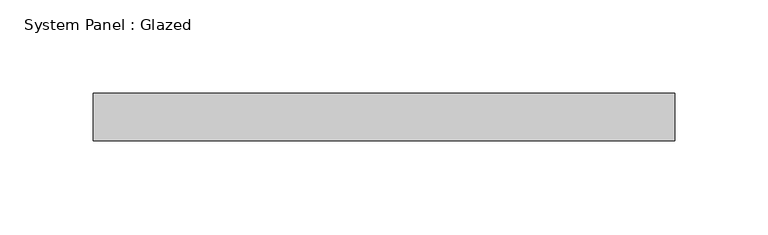
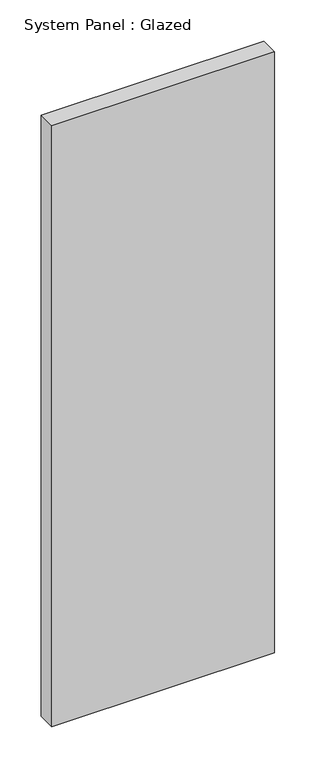
"""IFC4 building model written with IfcOpenShell, lengths in millimetres: plate geometry, System Panel : Glazed."""

from ifc_helpers import new_model, si_unit, origin, origin_with_axes, place, context, project, spatial, polyline, outline, extrude, source, transform, mapped, element, save


def system_panel_glazed_fcfd29d5(model_context):
    return source(origin(), model_context, "Body", "SweptSolid", [
        extrude(outline(polyline([(155.575, 19.05), (-155.575, 19.05), (-155.575, 44.45), (155.575, 44.45), (155.575, 19.05)])), origin_with_axes(), (0.0, 0.0, 1.0), 886.8833333),
    ])


if __name__ == "__main__":
    model = new_model("IFC4")
    model_context = context("Model", 3, world=origin())
    ifc_project = project(units=[si_unit("LENGTHUNIT", "METRE", prefix="MILLI")], contexts=[model_context])
    site = spatial("IfcSite", under=ifc_project)
    building = spatial("IfcBuilding", under=site)
    placement = place(None, origin())
    system_panel_glazed_shape = system_panel_glazed_fcfd29d5(model_context)
    element("IfcPlate", 1, ObjectType="System Panel : Glazed", at=placement, inside=building, context=model_context, shape_type="MappedRepresentation", body=[
        mapped(system_panel_glazed_shape, transform((0.0, 0.0, 0.0), x_axis=(1.0, 0.0, 0.0), y_axis=(0.0, 1.0, 0.0), z_axis=(0.0, 0.0, 1.0))),
    ])
    save(model, "model.ifc")

# Revit data of these elements
# Type "System Panel : Glazed"
#   Construction Type Id = "GSP4R"
#   Analytic Construction = "1/8 in Pilkington single glazing"
#   Visual Light Transmittance = 0.9
#   Solar Heat Gain Coefficient = 0.86
#   Heat Transfer Coefficient (U) = 1.18115 BTU/(h·ft²·°F)
# Element 1 (IfcPlate, "System Panel : Glazed")
#   Materials on its faces: "Glass"
# Materials
#   "Glass": class "Glass", colour RGB 0 128 192, transparency 0.75, Description = "Soda Lime Glass", Cost = 0
